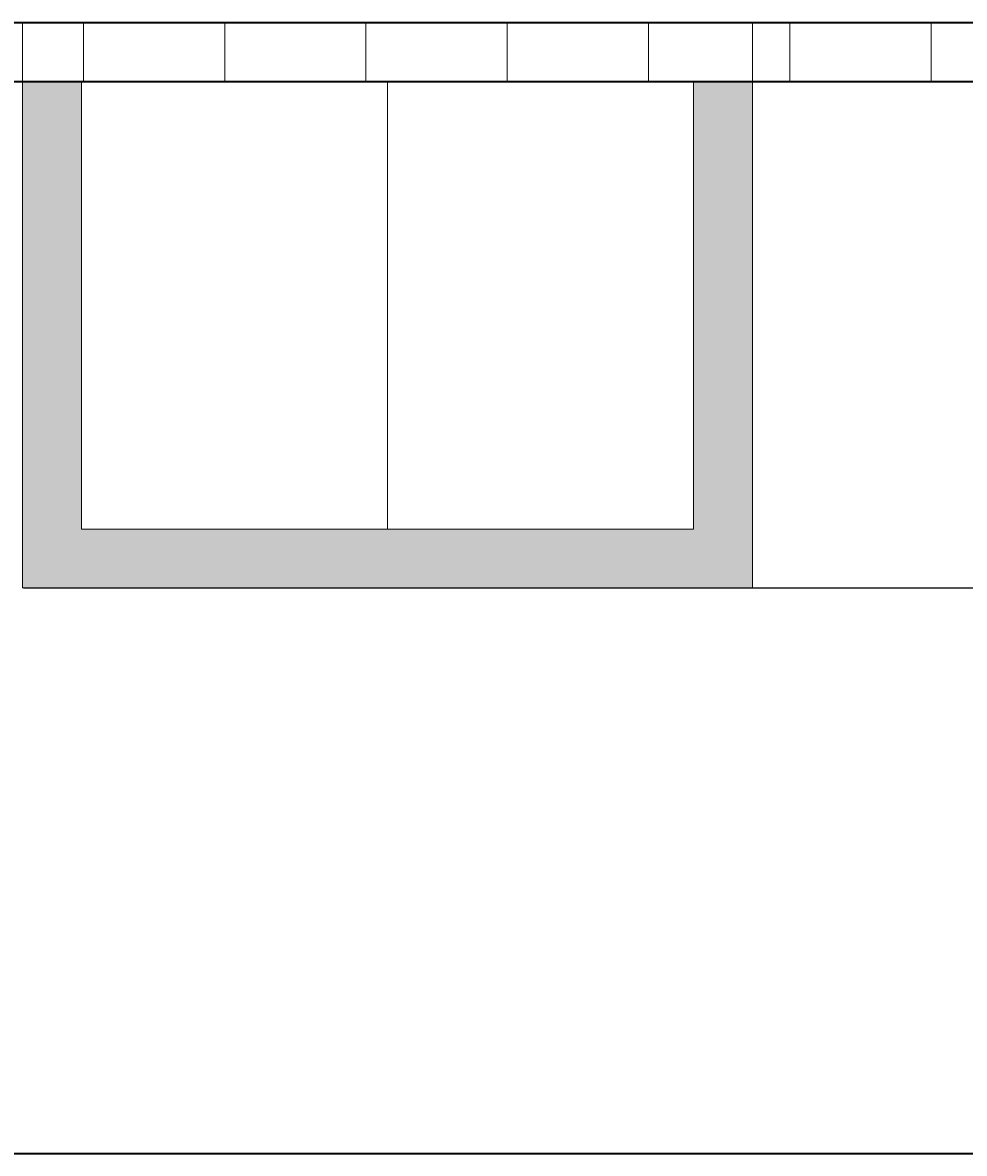
# Model space of a CAD drawing. Units: inches. Extents: x -128 to 854, y -395 to 398.
# Tile 15 of 61: x 199 to 279, y -298 to -202. Entities that reach past the tile are written whole.
import ezdxf

# ---------------------------------------------------------------- set-up
doc = ezdxf.new("R2010")
doc.units = ezdxf.units.IN
doc.header["$MEASUREMENT"] = 0
for name, color, linetype, lineweight in [('A-ANNO-DIMS', 2, 'Continuous', 18), ('A-GLAZ', 220, 'Continuous', 18), ('A-SECT', 220, 'Continuous', 35), ('A-SECT-PATT', 8, 'Continuous', 13)]:
    doc.layers.add(name, color=color, linetype=linetype, lineweight=lineweight)
doc.styles.get("Standard").update_dxf_attribs({"font": 'arial.ttf'})
doc.dimstyles.get("Standard").update_dxf_attribs({"dimtxt": 0.18, "dimasz": 0.18, "dimexe": 0.18, "dimexo": 0.0625, "dimgap": 0.09, "dimtad": 0, "dimtih": 1, "dimtoh": 1, "dimdec": 1, "dimzin": 0, "dimdsep": 46, "dimlunit": 4, "dimtxsty": 'Standard', "dimcen": 0.09, "dimclrd": 1, "dimclre": 2, "dimclrt": 6, "dimadec": 0, "dimazin": 0, "dimtfac": 1, "dimtdec": 1, "dimtofl": 0, "dimtmove": 0, "dimatfit": 3, "dimfxl": 1, "dimtfill": 2, "dimtfillclr": 3, "dimtolj": 1, "dimtzin": 0, "dimarcsym": 0})

# ---------------------------------------------------------------- blocks, each defined once
blk = doc.blocks.new('*D127')
at = {"layer": 'A-ANNO-DIMS', "color": 2, "lineweight": -2, "transparency": 16777216}
for p, q in [((260.902, -202.019), (389.719, -202.019)), ((317.902, -298.019), (389.719, -298.019))]:
    blk.add_line(p, q, dxfattribs=at)
at = {"layer": 'A-ANNO-DIMS', "color": 1, "lineweight": -2, "transparency": 16777216}
for p, q in [((389.539, -202.199), (389.539, -249.837)), ((389.539, -297.839), (389.539, -250.201))]:
    blk.add_line(p, q, dxfattribs=at)
at = {"layer": 'A-ANNO-DIMS', "color": 1, "transparency": 16777216}
for points in [[(389.509, -202.199), (389.569, -202.199), (389.539, -202.019)], [(389.509, -297.839), (389.569, -297.839), (389.539, -298.019)]]:
    blk.add_solid(points, dxfattribs=at)
at = {"layer": 'Defpoints', "color": 0, "transparency": 16777216}
for p in [(260.839, -202.019), (389.539, -202.019), (317.839, -298.019)]:
    blk.add_point(p, dxfattribs=at)
at = {"layer": 'A-ANNO-DIMS', "color": 6, "transparency": 16777216, "insert": (389.539, -250.019), "char_height": 0.18, "attachment_point": 5, "bg_fill": 1, "box_fill_scale": 1.25, "bg_fill_color": 3, "bg_fill_transparency": 0}
blk.add_mtext('\\A1;8\'-0"', dxfattribs=at)
blk = doc.blocks.new('*D132')
at = {"layer": 'A-ANNO-DIMS', "color": 2, "lineweight": -2, "transparency": 16777216}
for p, q in [((198.902, -250.019), (389.719, -250.019)), ((160.902, -298.019), (389.719, -298.019))]:
    blk.add_line(p, q, dxfattribs=at)
at = {"layer": 'A-ANNO-DIMS', "color": 1, "lineweight": -2, "transparency": 16777216}
for p, q in [((389.539, -250.199), (389.539, -273.837)), ((389.539, -297.839), (389.539, -274.201))]:
    blk.add_line(p, q, dxfattribs=at)
at = {"layer": 'A-ANNO-DIMS', "color": 1, "transparency": 16777216}
for points in [[(389.509, -250.199), (389.569, -250.199), (389.539, -250.019)], [(389.509, -297.839), (389.569, -297.839), (389.539, -298.019)]]:
    blk.add_solid(points, dxfattribs=at)
at = {"layer": 'Defpoints', "color": 0, "transparency": 16777216}
for p in [(198.839, -250.019), (389.539, -250.019), (160.839, -298.019)]:
    blk.add_point(p, dxfattribs=at)
at = {"layer": 'A-ANNO-DIMS', "color": 6, "transparency": 16777216, "insert": (389.539, -274.019), "char_height": 0.18, "attachment_point": 5, "bg_fill": 1, "box_fill_scale": 1.25, "bg_fill_color": 3, "bg_fill_transparency": 0}
blk.add_mtext('\\A1;4\'-0"', dxfattribs=at)

msp = doc.modelspace()

# ---------------------------------------------------------------- hatches: boundary and pattern name
at = {"layer": 'A-SECT-PATT'}
h = msp.add_hatch(dxfattribs=at)
h.set_pattern_fill('ANSI31', color=256, scale=96, angle=45, style=0)
h.paths.add_polyline_path([(-38.361, -202.019), (300.039, -202.019), (300.039, -207.019), (-38.361, -207.019)])
h = msp.add_hatch(color=256, dxfattribs=at)
h.dxf.hatch_style = 1
h.paths.add_polyline_path([(203.839, -207.019), (198.839, -207.019), (198.839, -250.019), (260.839, -250.019), (260.839, -207.019), (255.839, -207.019), (255.839, -245.019), (203.839, -245.019)])

# ---------------------------------------------------------------- linework, layer by layer
at = {"layer": 'A-GLAZ'}
msp.add_line((229.839, -207.019), (229.839, -245.019), dxfattribs=at)
for points in [[(198.839, -202.019), (260.839, -202.019), (260.839, -250.019), (198.839, -250.019)], [(203.839, -207.019), (255.839, -207.019), (255.839, -245.019), (203.839, -245.019)]]:
    msp.add_lwpolyline(points, close=True, dxfattribs=at)
at = {"layer": 'A-SECT'}
for p, q in [((-56.161, -202.019), (317.839, -202.019)), ((-56.161, -207.019), (317.839, -207.019)), ((-56.161, -298.019), (312.839, -298.019))]:
    msp.add_line(p, q, dxfattribs=at)

# ---------------------------------------------------------------- dimensions: what is measured, and where the dimension line sits
at = {"layer": 'A-ANNO-DIMS'}
for base, p1, p2, picture, middle in [((389.539, -202.019), (317.839, -298.019), (260.839, -202.019), '*D127', (389.539, -250.019)), ((389.539, -250.019), (160.839, -298.019), (198.839, -250.019), '*D132', (389.539, -274.019))]:
    dim = msp.add_linear_dim(base=base, p1=p1, p2=p2, angle=90, dimstyle='Standard', override={"dimdec": 1, "dimlfac": 1, "dimrnd": 0, "dimzin": 1, "dimdsep": 46, "dimlunit": 4, "dimfrac": 2}, dxfattribs=at)
    dim.commit()
    dim.dimension.update_dxf_attribs({"geometry": picture, "text_midpoint": middle})

doc.saveas('drawing.dxf')
